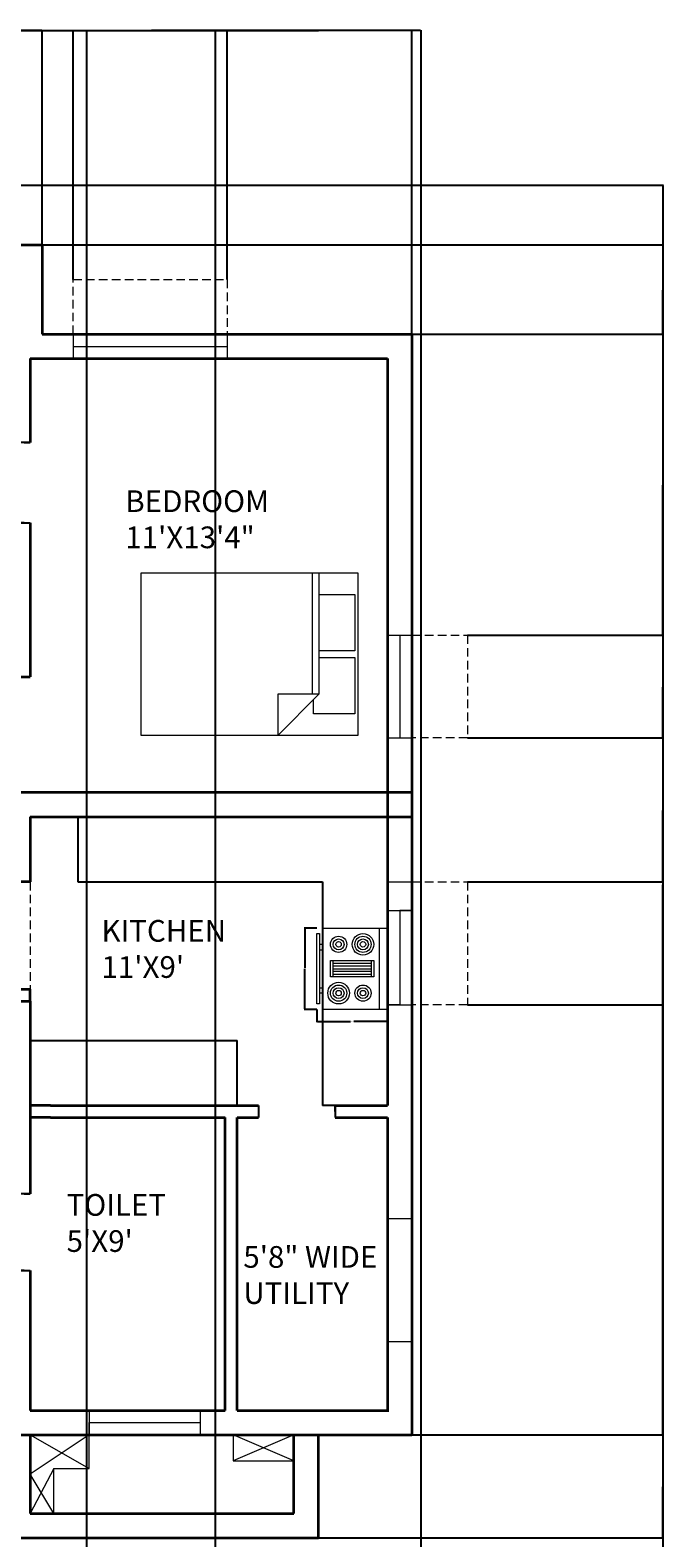
# Model space of a CAD drawing. Units: inches. Extents: x 276 to 912, y -567 to 621.
# Tile 7 of 7: x 678 to 912, y 65 to 621. Entities that reach past the tile are written whole.
import ezdxf

# ---------------------------------------------------------------- set-up
doc = ezdxf.new("R2010")
doc.units = ezdxf.units.IN
doc.linetypes.add('HIDDEN2', pattern=[4.7625, 3.175, -1.5875])
for name, color, linetype, lineweight in [('A-ANNO-DIMS', 2, 'Continuous', 18), ('A-AREA-IDEN', 7, 'Continuous', 18), ('A-DOOR', 3, 'Continuous', 25), ('A-EQPM', 9, 'Continuous', 18), ('A-FLOR-CASE', 9, 'Continuous', 25), ('A-FLOR-OVHD', 8, 'HIDDEN2', 13), ('A-FLOR-SHFT', 8, 'Continuous', 18), ('A-FURN', 8, 'Continuous', 18), ('A-GLAZ', 4, 'Continuous', 18), ('A-WALL', 7, 'Continuous', 35), ('A-WALL-HIDN', 8, 'HIDDEN2', 18)]:
    doc.layers.add(name, color=color, linetype=linetype, lineweight=lineweight)
doc.dimstyles.get("Standard").update_dxf_attribs({"dimtxt": 0.18, "dimasz": 0.18, "dimexe": 0.18, "dimexo": 0.0625, "dimgap": 0.09, "dimtad": 0, "dimtih": 1, "dimtoh": 1, "dimdec": 4, "dimzin": 0, "dimdsep": 46, "dimtxsty": 'Standard', "dimcen": 0.09, "dimadec": 0, "dimazin": 0, "dimtfac": 1, "dimtdec": 4, "dimtofl": 0, "dimtmove": 0, "dimatfit": 3, "dimfxl": 1, "dimtolj": 1, "dimtzin": 0, "dimarcsym": 0})

# ---------------------------------------------------------------- blocks, each defined once
blk = doc.blocks.new('Range-Oven - 30 in top')
for p, q in [((0, -3), (30, -3)), ((12, -6), (18, -6)), ((13, -20), (13, -6)), ((14, -6), (14, -20)), ((15, -20), (15, -6)), ((16, -6), (16, -20)), ((17, -20), (17, -6)), ((18, -20), (12, -20)), ((6, -24), (6, -25)), ((8, -25), (8, -24)), ((22, -25), (22, -24)), ((24, -24), (24, -25))]:
    blk.add_line(p, q)
for points in [[(0, -24), (0, 0), (30, 0), (30, -24)], [(12, -21), (12, -5), (18, -5), (18, -21)], [(2, -26), (2, -25), (28, -25), (28, -26)]]:
    blk.add_lwpolyline(points, close=True)
for centre, radius in [((6, -9), 4), ((6, -9), 3), ((6, -9), 2), ((6, -9), 1), ((24, -9), 3), ((24, -9), 2), ((24, -9), 1), ((6, -18), 3), ((6, -18), 2), ((24, -18), 4), ((24, -18), 3), ((24, -18), 2), ((6, -18), 1), ((24, -18), 1)]:
    blk.add_circle(centre, radius)
blk = doc.blocks.new('Bed - Queen')
for p, q in [((0, -80.00003), (0, 0)), ((0, 0), (59.99999, 0)), ((59.99999, 0), (59.99999, -80.00003)), ((7.99999, -1.2), (28.79998, -1.2)), ((7.99999, -14.4), (7.99999, -1.2)), ((28.79998, -1.2), (28.79998, -14.4)), ((31.19999, -1.2), (51.99999, -1.2)), ((31.19999, -14.4), (31.19999, -1.2)), ((51.99999, -1.2), (51.99999, -16.4)), ((0, -14.4), (44.8, -14.4)), ((59.99999, -29.6), (44.8, -14.4)), ((44.8, -14.4), (44.8, -29.6)), ((51.99999, -16.4), (46.79936, -16.4)), ((44.8, -16.8), (0, -16.8)), ((44.8, -29.6), (59.99999, -29.6)), ((59.99999, -80.00003), (0, -80.00003))]:
    blk.add_line(p, q)
blk = doc.blocks.new('DOOR-JAMB-4.5IN')
for p, q in [((0, 2.25), (0, 4.5)), ((0, 4.5), (0, 0))]:
    blk.add_line(p, q)
blk = doc.blocks.new('*D16')
at = {"layer": 'A-ANNO-DIMS', "color": 0, "lineweight": -2, "transparency": 16777216}
for p, q in [((783.42, 290.24), (778.81, 290.24)), ((778.99, 290.06), (778.99, 275.42)), ((778.99, 260.42), (778.99, 275.06)), ((783.42, 260.24), (778.81, 260.24))]:
    blk.add_line(p, q, dxfattribs=at)
at = {"layer": 'A-ANNO-DIMS', "color": 0, "transparency": 16777216}
for points in [[(778.96, 290.06), (779.02, 290.06), (778.99, 290.24)], [(778.96, 260.42), (779.02, 260.42), (778.99, 260.24)]]:
    blk.add_solid(points, dxfattribs=at)
at = {"layer": 'Defpoints', "color": 0, "transparency": 16777216}
for p in [(783.49, 290.24), (778.99, 260.24), (783.49, 260.24)]:
    blk.add_point(p, dxfattribs=at)
at = {"layer": 'A-ANNO-DIMS', "color": 0, "transparency": 16777216, "insert": (778.99, 275.24), "char_height": 0.18, "attachment_point": 5}
blk.add_mtext('\\A1;RANGE 30 TYP.', dxfattribs=at)
blk = doc.blocks.new('*D17')
at = {"layer": 'A-ANNO-DIMS', "color": 0, "lineweight": -2, "transparency": 16777216}
for p, q in [((783.49, 260.18), (783.49, 255.56)), ((809.49, 260.18), (809.49, 255.56)), ((783.67, 255.74), (795.86, 255.74)), ((809.31, 255.74), (797.12, 255.74))]:
    blk.add_line(p, q, dxfattribs=at)
at = {"layer": 'A-ANNO-DIMS', "color": 0, "transparency": 16777216}
for points in [[(783.67, 255.77), (783.67, 255.71), (783.49, 255.74)], [(809.31, 255.77), (809.31, 255.71), (809.49, 255.74)]]:
    blk.add_solid(points, dxfattribs=at)
at = {"layer": 'Defpoints', "color": 0, "transparency": 16777216}
for p in [(783.49, 260.24), (809.49, 260.24), (809.49, 255.74)]:
    blk.add_point(p, dxfattribs=at)
at = {"layer": 'A-ANNO-DIMS', "color": 0, "transparency": 16777216, "insert": (796.49, 255.74), "char_height": 0.18, "attachment_point": 5}
blk.add_mtext('\\A1;26 TYP.', dxfattribs=at)
blk = doc.blocks.new('*D24')
at = {"layer": 'A-ANNO-DIMS', "color": 0, "lineweight": -2, "transparency": 16777216}
for p, q in [((333.082179, 103.255751), (333.082179, -553.223061)), ((854.209085, -327.604004), (854.209085, -553.223061)), ((333.262179, -553.043061), (593.255632, -553.043061)), ((854.029085, -553.043061), (594.035632, -553.043061))]:
    blk.add_line(p, q, dxfattribs=at)
at = {"layer": 'A-ANNO-DIMS', "color": 0, "transparency": 16777216}
for points in [[(333.262179, -553.013061), (333.262179, -553.073061), (333.082179, -553.043061)], [(854.029085, -553.013061), (854.029085, -553.073061), (854.209085, -553.043061)]]:
    blk.add_solid(points, dxfattribs=at)
at = {"layer": 'Defpoints', "color": 0, "transparency": 16777216}
for p in [(333.082179, 103.318251), (854.209085, -327.541504), (854.209085, -553.043061)]:
    blk.add_point(p, dxfattribs=at)
at = {"layer": 'A-ANNO-DIMS', "color": 0, "transparency": 16777216, "insert": (593.645632, -553.043061), "char_height": 0.18, "attachment_point": 5}
blk.add_mtext('\\A1;521.1', dxfattribs=at)
blk = doc.blocks.new('*D25')
at = {"layer": 'A-ANNO-DIMS', "color": 0, "lineweight": -2, "transparency": 16777216}
for p, q in [((478.5, 564.29), (911.39, 564.29)), ((911.21, 564.11), (911.21, 34.31)), ((911.21, -495.86), (911.21, 33.95)), ((582.98, -496.04), (911.39, -496.04))]:
    blk.add_line(p, q, dxfattribs=at)
at = {"layer": 'A-ANNO-DIMS', "color": 0, "transparency": 16777216}
for points in [[(911.18, 564.11), (911.24, 564.11), (911.21, 564.29)], [(911.18, -495.86), (911.24, -495.86), (911.21, -496.04)]]:
    blk.add_solid(points, dxfattribs=at)
at = {"layer": 'Defpoints', "color": 0, "transparency": 16777216}
for p in [(478.44, 564.29), (582.92, -496.04), (911.21, -496.04)]:
    blk.add_point(p, dxfattribs=at)
at = {"layer": 'A-ANNO-DIMS', "color": 0, "transparency": 16777216, "insert": (911.21, 34.13), "char_height": 0.18, "attachment_point": 5}
blk.add_mtext('\\A1;1060.3', dxfattribs=at)
blk = doc.blocks.new('*D28')
at = {"layer": 'A-ANNO-DIMS', "color": 0, "lineweight": -2, "transparency": 16777216}
for p, q in [((604.082179, 542.322551), (604.082179, 621.473746)), ((604.262179, 621.293746), (642.842179, 621.293746)), ((681.902179, 621.293746), (643.322179, 621.293746)), ((682.082179, 542.322551), (682.082179, 621.473746))]:
    blk.add_line(p, q, dxfattribs=at)
at = {"layer": 'A-ANNO-DIMS', "color": 0, "transparency": 16777216}
for points in [[(604.262179, 621.323746), (604.262179, 621.263746), (604.082179, 621.293746)], [(681.902179, 621.323746), (681.902179, 621.263746), (682.082179, 621.293746)]]:
    blk.add_solid(points, dxfattribs=at)
at = {"layer": 'Defpoints', "color": 0, "transparency": 16777216}
for p in [(682.082179, 621.293746), (604.082179, 542.260051), (682.082179, 542.260051)]:
    blk.add_point(p, dxfattribs=at)
at = {"layer": 'A-ANNO-DIMS', "color": 0, "transparency": 16777216, "insert": (643.082179, 621.293746), "char_height": 0.18, "attachment_point": 5}
blk.add_mtext('\\A1;78', dxfattribs=at)
blk = doc.blocks.new('*D29')
at = {"layer": 'A-ANNO-DIMS', "color": 0, "lineweight": -2, "transparency": 16777216}
for p, q in [((682.082179, 542.322551), (682.082179, 621.473746)), ((682.262179, 621.293746), (749.912179, 621.293746)), ((818.402179, 621.293746), (750.752179, 621.293746)), ((818.582179, 509.380751), (818.582179, 621.473746))]:
    blk.add_line(p, q, dxfattribs=at)
at = {"layer": 'A-ANNO-DIMS', "color": 0, "transparency": 16777216}
for points in [[(682.262179, 621.323746), (682.262179, 621.263746), (682.082179, 621.293746)], [(818.402179, 621.323746), (818.402179, 621.263746), (818.582179, 621.293746)]]:
    blk.add_solid(points, dxfattribs=at)
at = {"layer": 'Defpoints', "color": 0, "transparency": 16777216}
for p in [(818.582179, 621.293746), (682.082179, 542.260051), (818.582179, 509.318251)]:
    blk.add_point(p, dxfattribs=at)
at = {"layer": 'A-ANNO-DIMS', "color": 0, "transparency": 16777216, "insert": (750.332179, 621.293746), "char_height": 0.18, "attachment_point": 5}
blk.add_mtext('\\A1;136.5', dxfattribs=at)
blk = doc.blocks.new('*D30')
at = {"layer": 'A-ANNO-DIMS', "color": 0, "lineweight": -2, "transparency": 16777216}
for p, q in [((818.644679, 509.318251), (911.389085, 509.318251)), ((911.209085, 509.138251), (911.209085, 306.498251)), ((911.209085, 103.498251), (911.209085, 306.138251)), ((818.644679, 103.318251), (911.389085, 103.318251))]:
    blk.add_line(p, q, dxfattribs=at)
at = {"layer": 'A-ANNO-DIMS', "color": 0, "transparency": 16777216}
for points in [[(911.179085, 509.138251), (911.239085, 509.138251), (911.209085, 509.318251)], [(911.179085, 103.498251), (911.239085, 103.498251), (911.209085, 103.318251)]]:
    blk.add_solid(points, dxfattribs=at)
at = {"layer": 'Defpoints', "color": 0, "transparency": 16777216}
for p in [(818.582179, 509.318251), (818.582179, 103.318251), (911.209085, 103.318251)]:
    blk.add_point(p, dxfattribs=at)
at = {"layer": 'A-ANNO-DIMS', "color": 0, "transparency": 16777216, "insert": (911.209085, 306.318251), "char_height": 0.18, "attachment_point": 5}
blk.add_mtext('\\A1;406', dxfattribs=at)
blk = doc.blocks.new('*D35')
at = {"layer": 'A-ANNO-DIMS', "color": 0, "lineweight": -2, "transparency": 16777216}
for p, q in [((784.0623, 103.318251), (911.389085, 103.318251)), ((911.209085, 103.138251), (911.209085, 84.493453)), ((911.209085, 65.488655), (911.209085, 84.133453)), ((784.0623, 65.308655), (911.389085, 65.308655))]:
    blk.add_line(p, q, dxfattribs=at)
at = {"layer": 'A-ANNO-DIMS', "color": 0, "transparency": 16777216}
for points in [[(911.179085, 103.138251), (911.239085, 103.138251), (911.209085, 103.318251)], [(911.179085, 65.488655), (911.239085, 65.488655), (911.209085, 65.308655)]]:
    blk.add_solid(points, dxfattribs=at)
at = {"layer": 'Defpoints', "color": 0, "transparency": 16777216}
for p in [(783.9998, 103.318251), (911.209085, 103.318251), (783.9998, 65.308655)]:
    blk.add_point(p, dxfattribs=at)
at = {"layer": 'A-ANNO-DIMS', "color": 0, "transparency": 16777216, "insert": (911.209085, 84.313453), "char_height": 0.18, "attachment_point": 5}
blk.add_mtext('\\A1;38.01', dxfattribs=at)
blk = doc.blocks.new('*D36')
at = {"layer": 'A-ANNO-DIMS', "color": 0, "lineweight": -2, "transparency": 16777216}
for p, q in [((682.144679, 542.260051), (911.389085, 542.260051)), ((911.209085, 542.080051), (911.209085, 525.969151)), ((911.209085, 509.498251), (911.209085, 525.609151)), ((682.144679, 509.318251), (911.389085, 509.318251))]:
    blk.add_line(p, q, dxfattribs=at)
at = {"layer": 'A-ANNO-DIMS', "color": 0, "transparency": 16777216}
for points in [[(911.179085, 542.080051), (911.239085, 542.080051), (911.209085, 542.260051)], [(911.179085, 509.498251), (911.239085, 509.498251), (911.209085, 509.318251)]]:
    blk.add_solid(points, dxfattribs=at)
at = {"layer": 'Defpoints', "color": 0, "transparency": 16777216}
for p in [(682.082179, 542.260051), (682.082179, 509.318251), (911.209085, 509.318251)]:
    blk.add_point(p, dxfattribs=at)
at = {"layer": 'A-ANNO-DIMS', "color": 0, "transparency": 16777216, "insert": (911.209085, 525.789151), "char_height": 0.18, "attachment_point": 5}
blk.add_mtext('\\A1;32.94', dxfattribs=at)
blk = doc.blocks.new('*D46')
at = {"layer": 'A-ANNO-DIMS', "color": 0, "lineweight": -2, "transparency": 16777216}
for p, q in [((693.468797, 529.52223), (693.468797, 621.473746)), ((693.648797, 621.293746), (721.450488, 621.293746)), ((750.152179, 621.293746), (722.350488, 621.293746)), ((750.332179, 529.52223), (750.332179, 621.473746))]:
    blk.add_line(p, q, dxfattribs=at)
at = {"layer": 'A-ANNO-DIMS', "color": 0, "transparency": 16777216}
for points in [[(693.648797, 621.323746), (693.648797, 621.263746), (693.468797, 621.293746)], [(750.152179, 621.323746), (750.152179, 621.263746), (750.332179, 621.293746)]]:
    blk.add_solid(points, dxfattribs=at)
at = {"layer": 'Defpoints', "color": 0, "transparency": 16777216}
for p in [(750.332179, 621.293746), (693.468797, 529.45973), (750.332179, 529.45973)]:
    blk.add_point(p, dxfattribs=at)
at = {"layer": 'A-ANNO-DIMS', "color": 0, "transparency": 16777216, "insert": (721.900488, 621.293746), "char_height": 0.18, "attachment_point": 5}
blk.add_mtext('\\A1;56.86', dxfattribs=at)
blk = doc.blocks.new('*D47')
at = {"layer": 'A-ANNO-DIMS', "color": 0, "lineweight": -2, "transparency": 16777216}
for p, q in [((750.332179, 529.52223), (750.332179, 621.473746)), ((750.512179, 621.293746), (784.007179, 621.293746)), ((818.402179, 621.293746), (784.907179, 621.293746)), ((818.582179, 509.380751), (818.582179, 621.473746))]:
    blk.add_line(p, q, dxfattribs=at)
at = {"layer": 'A-ANNO-DIMS', "color": 0, "transparency": 16777216}
for points in [[(750.512179, 621.323746), (750.512179, 621.263746), (750.332179, 621.293746)], [(818.402179, 621.323746), (818.402179, 621.263746), (818.582179, 621.293746)]]:
    blk.add_solid(points, dxfattribs=at)
at = {"layer": 'Defpoints', "color": 0, "transparency": 16777216}
for p in [(818.582179, 621.293746), (750.332179, 529.45973), (818.582179, 509.318251)]:
    blk.add_point(p, dxfattribs=at)
at = {"layer": 'A-ANNO-DIMS', "color": 0, "transparency": 16777216, "insert": (784.457179, 621.293746), "char_height": 0.18, "attachment_point": 5}
blk.add_mtext('\\A1;68.25', dxfattribs=at)
blk = doc.blocks.new('*D48')
at = {"layer": 'A-ANNO-DIMS', "color": 0, "lineweight": -2, "transparency": 16777216}
for p, q in [((818.644679, 509.318251), (911.389085, 509.318251)), ((911.209085, 509.138251), (911.209085, 453.998251)), ((911.209085, 398.498251), (911.209085, 453.638251)), ((839.079588, 398.318251), (911.389085, 398.318251))]:
    blk.add_line(p, q, dxfattribs=at)
at = {"layer": 'A-ANNO-DIMS', "color": 0, "transparency": 16777216}
for points in [[(911.179085, 509.138251), (911.239085, 509.138251), (911.209085, 509.318251)], [(911.179085, 398.498251), (911.239085, 398.498251), (911.209085, 398.318251)]]:
    blk.add_solid(points, dxfattribs=at)
at = {"layer": 'Defpoints', "color": 0, "transparency": 16777216}
for p in [(818.582179, 509.318251), (839.017088, 398.318251), (911.209085, 398.318251)]:
    blk.add_point(p, dxfattribs=at)
at = {"layer": 'A-ANNO-DIMS', "color": 0, "transparency": 16777216, "insert": (911.209085, 453.818251), "char_height": 0.18, "attachment_point": 5}
blk.add_mtext('\\A1;111', dxfattribs=at)
blk = doc.blocks.new('*D49')
at = {"layer": 'A-ANNO-DIMS', "color": 0, "lineweight": -2, "transparency": 16777216}
for p, q in [((839.08, 398.32), (911.39, 398.32)), ((911.21, 398.14), (911.21, 379.52)), ((911.21, 360.54), (911.21, 379.16)), ((839.08, 360.36), (911.39, 360.36))]:
    blk.add_line(p, q, dxfattribs=at)
at = {"layer": 'A-ANNO-DIMS', "color": 0, "transparency": 16777216}
for points in [[(911.18, 398.14), (911.24, 398.14), (911.21, 398.32)], [(911.18, 360.54), (911.24, 360.54), (911.21, 360.36)]]:
    blk.add_solid(points, dxfattribs=at)
at = {"layer": 'Defpoints', "color": 0, "transparency": 16777216}
for p in [(839.02, 398.32), (839.02, 360.36), (911.21, 360.36)]:
    blk.add_point(p, dxfattribs=at)
at = {"layer": 'A-ANNO-DIMS', "color": 0, "transparency": 16777216, "insert": (911.21, 379.34), "char_height": 0.18, "attachment_point": 5}
blk.add_mtext('\\A1;37.954', dxfattribs=at)
blk = doc.blocks.new('*D50')
at = {"layer": 'A-ANNO-DIMS', "color": 0, "lineweight": -2, "transparency": 16777216}
for p, q in [((839.08, 360.36), (911.39, 360.36)), ((911.21, 360.18), (911.21, 334.02)), ((911.21, 307.5), (911.21, 333.66)), ((839.08, 307.32), (911.39, 307.32))]:
    blk.add_line(p, q, dxfattribs=at)
at = {"layer": 'A-ANNO-DIMS', "color": 0, "transparency": 16777216}
for points in [[(911.18, 360.18), (911.24, 360.18), (911.21, 360.36)], [(911.18, 307.5), (911.24, 307.5), (911.21, 307.32)]]:
    blk.add_solid(points, dxfattribs=at)
at = {"layer": 'Defpoints', "color": 0, "transparency": 16777216}
for p in [(839.02, 360.36), (839.02, 307.32), (911.21, 307.32)]:
    blk.add_point(p, dxfattribs=at)
at = {"layer": 'A-ANNO-DIMS', "color": 0, "transparency": 16777216, "insert": (911.21, 333.84), "char_height": 0.18, "attachment_point": 5}
blk.add_mtext('\\A1;53.05', dxfattribs=at)
blk = doc.blocks.new('*D51')
at = {"layer": 'A-ANNO-DIMS', "color": 0, "lineweight": -2, "transparency": 16777216}
for p, q in [((839.079588, 307.318251), (911.389085, 307.318251)), ((911.209085, 307.138251), (911.209085, 284.790639)), ((911.209085, 262.083027), (911.209085, 284.430639)), ((839.079588, 261.903027), (911.389085, 261.903027))]:
    blk.add_line(p, q, dxfattribs=at)
at = {"layer": 'A-ANNO-DIMS', "color": 0, "transparency": 16777216}
for points in [[(911.179085, 307.138251), (911.239085, 307.138251), (911.209085, 307.318251)], [(911.179085, 262.083027), (911.239085, 262.083027), (911.209085, 261.903027)]]:
    blk.add_solid(points, dxfattribs=at)
at = {"layer": 'Defpoints', "color": 0, "transparency": 16777216}
for p in [(839.017088, 307.318251), (839.017088, 261.903027), (911.209085, 261.903027)]:
    blk.add_point(p, dxfattribs=at)
at = {"layer": 'A-ANNO-DIMS', "color": 0, "transparency": 16777216, "insert": (911.209085, 284.610639), "char_height": 0.18, "attachment_point": 5}
blk.add_mtext('\\A1;45.415', dxfattribs=at)
blk = doc.blocks.new('*D61')
at = {"layer": 'A-ANNO-DIMS', "color": 0, "lineweight": -2, "transparency": 16777216}
for p, q in [((661.418489, -30.671128), (661.418489, 621.473746)), ((661.598489, 621.293746), (741.263489, 621.293746)), ((821.738489, 621.293746), (742.073489, 621.293746)), ((821.918489, -64.479004), (821.918489, 621.473746))]:
    blk.add_line(p, q, dxfattribs=at)
at = {"layer": 'A-ANNO-DIMS', "color": 0, "transparency": 16777216}
for points in [[(661.598489, 621.323746), (661.598489, 621.263746), (661.418489, 621.293746)], [(821.738489, 621.323746), (821.738489, 621.263746), (821.918489, 621.293746)]]:
    blk.add_solid(points, dxfattribs=at)
at = {"layer": 'Defpoints', "color": 0, "transparency": 16777216}
for p in [(821.918489, 621.293746), (661.418489, -30.733628), (821.918489, -64.541504)]:
    blk.add_point(p, dxfattribs=at)
at = {"layer": 'A-ANNO-DIMS', "color": 0, "transparency": 16777216, "insert": (741.668489, 621.293746), "char_height": 0.18, "attachment_point": 5}
blk.add_mtext('\\A1;160.5', dxfattribs=at)
blk = doc.blocks.new('*D72')
at = {"layer": 'A-ANNO-DIMS', "color": 0, "lineweight": -2, "transparency": 16777216}
for p, q in [((698.51, -43.28), (698.51, 621.47)), ((698.69, 621.29), (721.9, 621.29)), ((745.83, 621.29), (722.62, 621.29)), ((746.01, -43.28), (746.01, 621.47))]:
    blk.add_line(p, q, dxfattribs=at)
at = {"layer": 'A-ANNO-DIMS', "color": 0, "transparency": 16777216}
for points in [[(698.69, 621.32), (698.69, 621.26), (698.51, 621.29)], [(745.83, 621.32), (745.83, 621.26), (746.01, 621.29)]]:
    blk.add_solid(points, dxfattribs=at)
at = {"layer": 'Defpoints', "color": 0, "transparency": 16777216}
for p in [(746.01, 621.29), (698.51, -43.34), (746.01, -43.34)]:
    blk.add_point(p, dxfattribs=at)
at = {"layer": 'A-ANNO-DIMS', "color": 0, "transparency": 16777216, "insert": (722.26, 621.29), "char_height": 0.18, "attachment_point": 5}
blk.add_mtext('\\A1;47.5', dxfattribs=at)
blk = doc.blocks.new('*D73')
at = {"layer": 'A-ANNO-DIMS', "color": 0, "lineweight": -2, "transparency": 16777216}
for p, q in [((746.01, -43.28), (746.01, 621.47)), ((746.19, 621.29), (783.61, 621.29)), ((821.74, 621.29), (784.33, 621.29)), ((821.92, -64.48), (821.92, 621.47))]:
    blk.add_line(p, q, dxfattribs=at)
at = {"layer": 'A-ANNO-DIMS', "color": 0, "transparency": 16777216}
for points in [[(746.19, 621.32), (746.19, 621.26), (746.01, 621.29)], [(821.74, 621.32), (821.74, 621.26), (821.92, 621.29)]]:
    blk.add_solid(points, dxfattribs=at)
at = {"layer": 'Defpoints', "color": 0, "transparency": 16777216}
for p in [(821.92, 621.29), (746.01, -43.34), (821.92, -64.54)]:
    blk.add_point(p, dxfattribs=at)
at = {"layer": 'A-ANNO-DIMS', "color": 0, "transparency": 16777216, "insert": (783.97, 621.29), "char_height": 0.18, "attachment_point": 5}
blk.add_mtext('\\A1;75.9', dxfattribs=at)

msp = doc.modelspace()

# ---------------------------------------------------------------- linework, layer by layer
at = {"layer": 'A-DOOR'}
msp.add_line((761.8684, 224.8183), (761.8684, 220.3183), dxfattribs=at)
at = {"layer": 'A-FLOR-CASE'}
for p, q in [((695.1704, 331.3183), (695.1704, 307.3183)), ((695.1704, 307.3183), (785.5822, 307.3183)), ((785.5822, 307.3183), (785.5822, 224.8183)), ((677.5822, 248.8183), (754.0822, 248.8183)), ((754.0822, 224.8183), (754.0822, 248.8183)), ((790.1541, 224.8183), (785.5822, 224.8183))]:
    msp.add_line(p, q, dxfattribs=at)
at = {"layer": 'A-FLOR-OVHD'}
for p, q in [((693.4688, 509.3183), (693.4688, 529.4597)), ((693.4688, 529.4597), (750.3322, 529.4597)), ((750.3322, 529.4597), (750.3322, 509.3183)), ((818.5822, 398.3183), (839.0171, 398.3183)), ((839.0171, 398.3183), (839.0171, 360.3644)), ((839.0171, 360.3644), (818.5822, 360.3644)), ((818.5822, 307.3183), (839.0171, 307.3183)), ((839.0171, 307.3183), (839.0171, 261.903)), ((839.0171, 261.903), (818.5822, 261.903))]:
    msp.add_line(p, q, dxfattribs=at)
at = {"layer": 'A-FLOR-SHFT'}
for p, q in [((699.3313, 103.3183), (677.5822, 88.8135)), ((677.5822, 103.3183), (699.3313, 90.8753)), ((699.3313, 90.8753), (699.3313, 103.3183)), ((752.5256, 103.3183), (752.5256, 93.7527)), ((774.9998, 93.7527), (752.5256, 103.3183)), ((774.9998, 103.3183), (752.5256, 93.7527)), ((686.3227, 90.8753), (677.5822, 74.3087)), ((686.3227, 74.3087), (686.3227, 90.8753)), ((686.3227, 90.8753), (699.3313, 90.8753)), ((752.5256, 93.7527), (774.9998, 93.7527)), ((686.3227, 74.3087), (677.5822, 88.8135))]:
    msp.add_line(p, q, dxfattribs=at)
at = {"layer": 'A-GLAZ'}
for p, q in [((693.4688, 509.3183), (693.4688, 500.3183)), ((750.3322, 509.3183), (750.3322, 500.3183)), ((693.4688, 504.8183), (750.3322, 504.8183)), ((750.3322, 500.3183), (750.3322, 500.3183)), ((809.5822, 398.3183), (818.5822, 398.3183)), ((814.0822, 398.3183), (814.0822, 360.3644)), ((809.5822, 360.3644), (818.5822, 360.3644)), ((809.5822, 307.3183), (818.5822, 307.3183)), ((809.5822, 296.7373), (818.5822, 296.7373)), ((818.5822, 296.7373), (814.0822, 296.7373)), ((814.0822, 296.7373), (814.0822, 261.903)), ((814.0822, 261.903), (809.5822, 261.903)), ((809.5822, 261.903), (818.5822, 261.903)), ((809.5822, 183.0928), (818.5822, 183.0928)), ((809.5822, 137.7974), (818.5822, 137.7974)), ((699.3313, 112.3183), (699.3313, 103.3183)), ((740.3712, 112.3183), (740.3712, 103.3183)), ((699.3313, 103.3183), (699.3313, 107.8183)), ((699.3313, 107.8183), (740.3712, 107.8183))]:
    msp.add_line(p, q, dxfattribs=at)
at = {"layer": 'A-WALL'}
for p, q in [((604.0822, 542.2601), (682.0822, 542.2601)), ((682.0822, 542.2601), (682.0822, 509.3183)), ((682.0822, 509.3183), (818.5822, 509.3183)), ((818.5822, 509.3183), (818.5822, 432.3183)), ((677.5822, 500.3183), (677.5822, 469.3985)), ((677.5822, 500.3183), (809.5822, 500.3183)), ((809.5822, 500.3183), (809.5822, 432.3183)), ((677.5822, 439.7271), (677.5822, 432.3183)), ((677.5822, 432.3183), (677.5822, 382.9782)), ((809.5822, 432.3183), (809.5822, 224.8183)), ((818.5822, 432.3183), (818.5822, 103.3183)), ((673.0822, 382.9782), (677.5822, 382.9782)), ((673.0822, 340.3183), (818.5822, 340.3183)), ((677.5822, 331.3183), (818.5822, 331.3183)), ((677.5822, 331.3183), (677.5822, 307.3183)), ((677.5822, 307.3183), (673.0822, 307.3183)), ((673.0822, 267.7214), (677.5822, 267.7214)), ((677.5822, 263.2214), (677.5822, 267.7214)), ((673.0822, 263.2214), (677.5822, 263.2214)), ((677.5822, 263.2214), (677.5822, 192.2677)), ((685.0822, 224.8183), (677.5822, 224.8183)), ((685.0822, 224.8183), (761.8684, 224.8183)), ((790.1541, 224.8183), (809.5822, 224.8183)), ((685.0822, 220.3183), (677.5822, 220.3183)), ((685.0822, 220.3183), (749.5822, 220.3183)), ((749.5822, 112.3183), (749.5822, 220.3183)), ((754.0822, 112.3183), (754.0822, 220.3183)), ((754.0822, 220.3183), (761.8684, 220.3183)), ((790.1541, 220.3183), (809.5822, 220.3183)), ((809.5822, 220.3183), (809.5822, 112.3183)), ((677.5822, 163.8902), (677.5822, 112.3183)), ((677.5822, 112.3183), (749.5822, 112.3183)), ((754.0822, 112.3183), (810.0822, 112.3183)), ((342.0822, 103.3183), (818.5822, 103.3183)), ((677.5822, 103.3183), (677.5822, 74.3087)), ((774.9998, 74.3087), (774.9998, 103.3183)), ((783.9998, 65.3087), (783.9998, 103.3183)), ((677.5822, 74.3087), (774.9998, 74.3087)), ((668.5822, 65.3087), (783.9998, 65.3087))]:
    msp.add_line(p, q, dxfattribs=at)
at = {"layer": 'A-WALL-HIDN'}
msp.add_line((677.5822, 307.3183), (677.5822, 267.7214), dxfattribs=at)

# ---------------------------------------------------------------- block references
at = {"layer": 'A-DOOR'}
for p, rotation in [((673.0819, 469.3985), 270), ((677.5824, 439.727), 90), ((673.0819, 192.2678), 270), ((677.5824, 163.8901), 90)]:
    msp.add_blockref('DOOR-JAMB-4.5IN', p, dxfattribs=dict(at, rotation=rotation))
msp.add_blockref('DOOR-JAMB-4.5IN', (790.154, 220.318), dxfattribs=at)
at = {"layer": 'A-EQPM', "rotation": 270}
msp.add_blockref('Range-Oven - 30 in top', (809.4869, 290.2448), dxfattribs=at)
at = {"layer": 'A-FURN', "rotation": 270}
msp.add_blockref('Bed - Queen', (798.6162, 421.2901), dxfattribs=at)

# ---------------------------------------------------------------- texts
at = {"layer": 'A-AREA-IDEN', "char_height": 8, "attachment_point": 1}
for s, insert in [('{\\fTimes New Roman|b0|i0|c0|p18;BEDROOM\\P11\'X13\'4"}', (712.7157, 451.7156)), ("{\\fTimes New Roman|b0|i0|c0|p18;KITCHEN\\P11'X9'}", (703.9333, 293.2174)), ("{\\fTimes New Roman|b0|i0|c0|p18;TOILET\\P5'X9'}", (691.052, 192.1281)), ('{\\fTimes New Roman|b0|i0|c0|p18;5\'8" WIDE UTILITY}', (756.3082, 172.9339))]:
    msp.add_mtext_dynamic_manual_height_columns(s, width=62.274017, gutter_width=12.5, heights=[0], dxfattribs=dict(at, insert=insert))

# ---------------------------------------------------------------- dimensions: what is measured, and where the dimension line sits
at = {"layer": 'A-ANNO-DIMS'}
for base, p1, p2, override, picture, middle in [((682.0822, 621.2937), (604.0822, 542.2601), (682.0822, 542.2601), {"dimdec": 0, "dimlfac": 1, "dimrnd": 0, "dimzin": 0, "dimdsep": 46, "dimlunit": 2}, '*D28', (643.0822, 621.2937)), ((821.9185, 621.2937), (661.4185, -30.7336), (821.9185, -64.5415), {"dimdec": 1, "dimlfac": 1, "dimrnd": 0, "dimzin": 0, "dimdsep": 46, "dimlunit": 2}, '*D61', (741.6685, 621.2937)), ((818.5822, 621.2937), (682.0822, 542.2601), (818.5822, 509.3183), {"dimdec": 1, "dimlfac": 1, "dimrnd": 0, "dimzin": 0, "dimdsep": 46, "dimlunit": 2}, '*D29', (750.3322, 621.2937)), ((750.3322, 621.2937), (693.4688, 529.4597), (750.3322, 529.4597), {"dimdec": 2, "dimlfac": 1, "dimrnd": 0, "dimzin": 0, "dimdsep": 46, "dimlunit": 2}, '*D46', (721.9005, 621.2937)), ((746.0116, 621.2937), (698.5118, -43.3384), (746.0116, -43.3384), {"dimdec": 1, "dimlfac": 1, "dimrnd": 0, "dimzin": 0, "dimdsep": 46, "dimlunit": 2}, '*D72', (722.2617, 621.2937)), ((821.9185, 621.2937), (746.0116, -43.3384), (821.9185, -64.5415), {"dimdec": 1, "dimlfac": 1, "dimrnd": 0, "dimzin": 0, "dimdsep": 46, "dimlunit": 2}, '*D73', (783.9651, 621.2937)), ((818.5822, 621.2937), (750.3322, 529.4597), (818.5822, 509.3183), {"dimdec": 2, "dimlfac": 1, "dimrnd": 0, "dimzin": 0, "dimdsep": 46, "dimlunit": 2}, '*D47', (784.4572, 621.2937)), ((854.2091, -553.0431), (333.0822, 103.3183), (854.2091, -327.5415), {"dimdec": 1, "dimlfac": 1, "dimrnd": 0, "dimzin": 0, "dimdsep": 46, "dimlunit": 2}, '*D24', (593.6456, -553.0431))]:
    dim = msp.add_linear_dim(base=base, p1=p1, p2=p2, dimstyle='Standard', override=override, dxfattribs=at)
    dim.commit()
    dim.dimension.update_dxf_attribs({"geometry": picture, "text_midpoint": middle})
for base, p1, p2, override, picture, middle in [((911.2091, -496.0431), (478.4357, 564.2937), (582.9185, -496.0431), {"dimdec": 1, "dimlfac": 1, "dimrnd": 0, "dimzin": 0, "dimdsep": 46, "dimlunit": 2}, '*D25', (911.2091, 34.1253)), ((911.2091, 509.3183), (682.0822, 542.2601), (682.0822, 509.3183), {"dimdec": 2, "dimlfac": 1, "dimrnd": 0, "dimzin": 0, "dimdsep": 46, "dimlunit": 2}, '*D36', (911.2091, 525.7892)), ((911.2091, 103.3183), (818.5822, 509.3183), (818.5822, 103.3183), {"dimdec": 0, "dimlfac": 1, "dimrnd": 0, "dimzin": 0, "dimdsep": 46, "dimlunit": 2}, '*D30', (911.2091, 306.3183)), ((911.2091, 398.3183), (818.5822, 509.3183), (839.0171, 398.3183), {"dimdec": 0, "dimlfac": 1, "dimrnd": 0, "dimzin": 0, "dimdsep": 46, "dimlunit": 2}, '*D48', (911.2091, 453.8183)), ((911.2091, 360.3644), (839.0171, 398.3183), (839.0171, 360.3644), {"dimdec": 3, "dimlfac": 1, "dimrnd": 0, "dimzin": 0, "dimdsep": 46, "dimlunit": 2}, '*D49', (911.2091, 379.3413)), ((911.2091, 307.3183), (839.0171, 360.3644), (839.0171, 307.3183), {"dimdec": 2, "dimlfac": 1, "dimrnd": 0, "dimzin": 0, "dimdsep": 46, "dimlunit": 2}, '*D50', (911.2091, 333.8413)), ((911.2091, 261.903), (839.0171, 307.3183), (839.0171, 261.903), {"dimdec": 3, "dimlfac": 1, "dimrnd": 0, "dimzin": 0, "dimdsep": 46, "dimlunit": 2}, '*D51', (911.2091, 284.6106)), ((911.2091, 103.3183), (783.9998, 65.3087), (783.9998, 103.3183), {"dimdec": 2, "dimlfac": 1, "dimrnd": 0, "dimzin": 0, "dimdsep": 46, "dimlunit": 2}, '*D35', (911.2091, 84.3135))]:
    dim = msp.add_linear_dim(base=base, p1=p1, p2=p2, angle=90, dimstyle='Standard', override=override, dxfattribs=at)
    dim.commit()
    dim.dimension.update_dxf_attribs({"geometry": picture, "text_midpoint": middle})
dim = msp.add_linear_dim(base=(778.9869, 260.2448), p1=(783.4869, 290.2448), p2=(783.4869, 260.2448), angle=270, text='RANGE <> TYP.', dimstyle='Standard', override={"dimdec": 0, "dimlfac": 1, "dimrnd": 0, "dimzin": 0, "dimdsep": 46, "dimlunit": 2}, dxfattribs=at)
dim.commit()
dim.dimension.update_dxf_attribs({"geometry": '*D16', "text_midpoint": (778.9869, 275.2448)})
dim = msp.add_linear_dim(base=(809.4869, 255.7448), p1=(783.4869, 260.2448), p2=(809.4869, 260.2448), text='<> TYP.', dimstyle='Standard', override={"dimdec": 0, "dimlfac": 1, "dimrnd": 0, "dimzin": 0, "dimdsep": 46, "dimlunit": 2}, dxfattribs=at)
dim.commit()
dim.dimension.update_dxf_attribs({"geometry": '*D17', "text_midpoint": (796.4869, 255.7448)})

doc.saveas('drawing.dxf')
